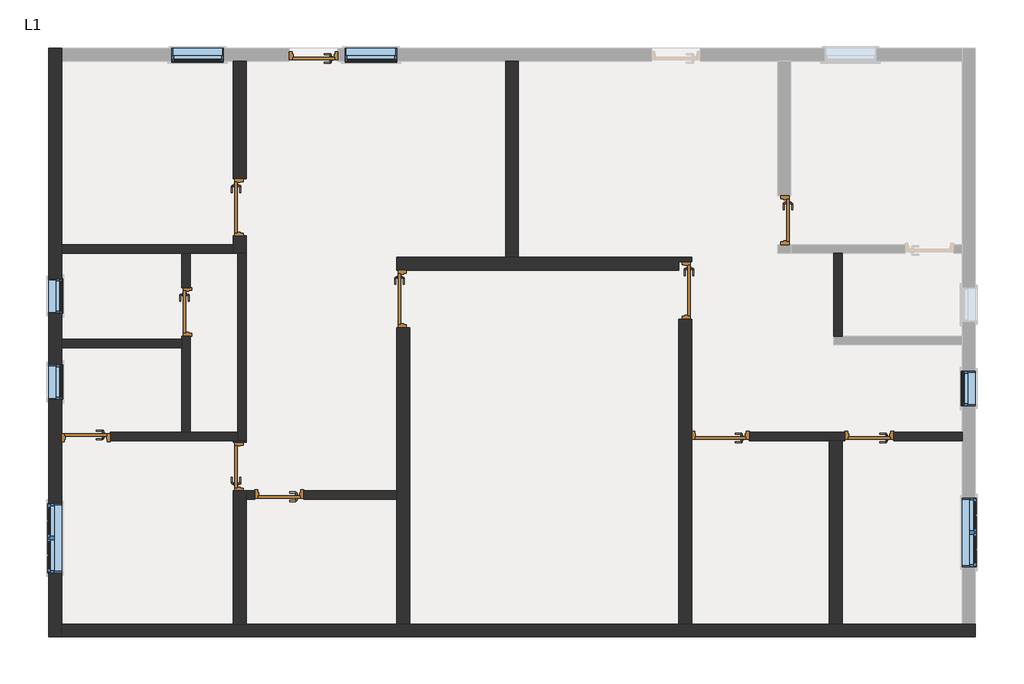
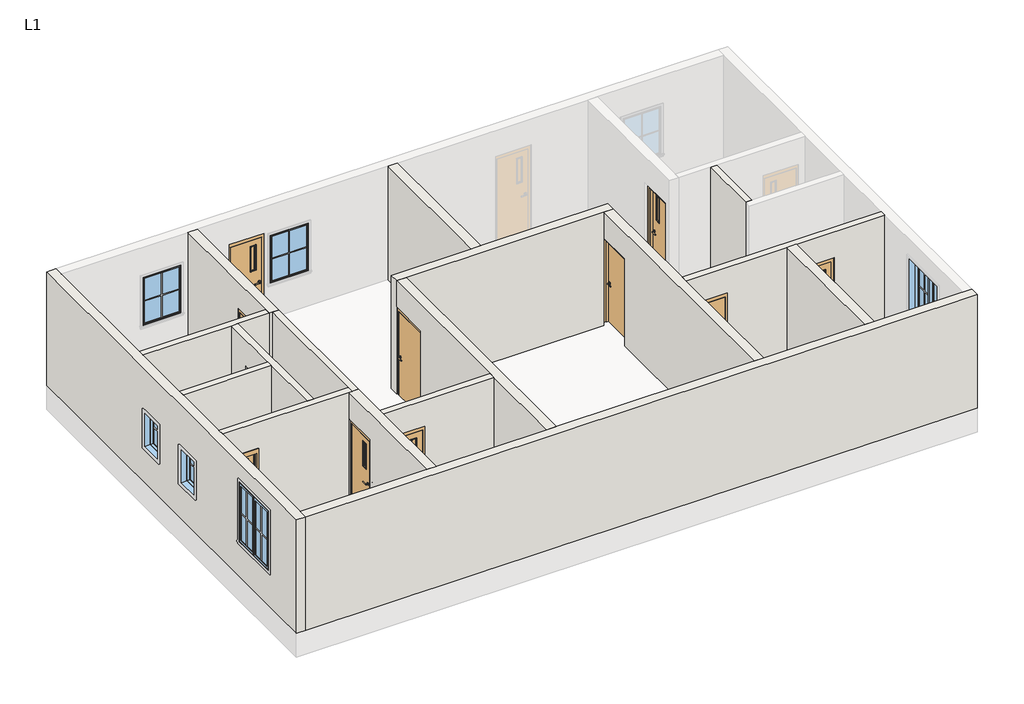
# One storey, part 1 of 2: 17 walls, 11 doors, 7 windows.
"""IFC4 building model written with IfcOpenShell, lengths in millimetres."""

from ifc_helpers import new_model, si_unit, frame, origin, place, context, project, spatial, polyline, outline, extrude, faceted_brep, transform, mapped, element, save
from components import door_9a5ad36a, door_70ceb761, door_9ff278b0, door_e76c17f4, door_2faac2b1, door_21b9ace8, window_8377141f, window_b8e47f08, window_2799360a

model = new_model("IFC4")

# Units and contexts
model_context = context("Model", 3, world=origin())
ifc_project = project(units=[si_unit("LENGTHUNIT", "METRE", prefix="MILLI")], contexts=[model_context])

# Site, building, storey
site = spatial("IfcSite", under=ifc_project)
building = spatial("IfcBuilding", under=site)
storey = spatial("IfcBuildingStorey", under=building, Name="L1", Elevation=609.6)

# Doors
placement = place(None, origin())
door_shape = door_9a5ad36a(model_context)
element("IfcDoor", 1, ObjectType="Door-Passage-Single-Flush : 36\" x 84\"", at=placement, inside=storey, context=model_context, shape_type="MappedRepresentation", body=[
    mapped(door_shape, transform((-2601.2379185, 2629.4278379, 609.6), x_axis=(0.0, -1.0, 0.0), y_axis=(1.0, 0.0, 0.0), z_axis=(0.0, 0.0, 1.0))),
])
element("IfcDoor", 2, ObjectType="Door-Passage-Single-Flush : 36\" x 84\"", at=placement, inside=storey, context=model_context, shape_type="MappedRepresentation", body=[
    mapped(door_shape, transform((294.3620815, 1003.8278379, 609.6), x_axis=(0.0, -1.0, 0.0), y_axis=(1.0, 0.0, 0.0), z_axis=(0.0, 0.0, 1.0))),
])
door_2_shape = door_70ceb761(model_context)
element("IfcDoor", 3, ObjectType="Door-Passage-Single-Flush : 36\" x 84\"", at=placement, inside=storey, context=model_context, shape_type="MappedRepresentation", body=[
    mapped(door_2_shape, transform((5914.1120815, -1428.2221621, 609.6), x_axis=(-1.0, 0.0, 0.0), y_axis=(0.0, -1.0, 0.0), z_axis=(0.0, 0.0, 1.0))),
])
door_3_shape = door_9ff278b0(model_context)
element("IfcDoor", 4, ObjectType="Door-Passage-Single-Flush : 36\" x 84\"", at=placement, inside=storey, context=model_context, shape_type="MappedRepresentation", body=[
    mapped(door_3_shape, transform((5285.4620815, 1156.2278379, 609.6), x_axis=(0.0, -1.0, 0.0), y_axis=(1.0, 0.0, 0.0), z_axis=(0.0, 0.0, 1.0))),
])
door_4_shape = door_e76c17f4(model_context)
element("IfcDoor", 5, ObjectType="Door-Passage-Single-Vision_Lite : 30\" x 84\"", at=placement, inside=storey, context=model_context, shape_type="MappedRepresentation", body=[
    mapped(door_4_shape, transform((-2601.2379185, -1967.9721621, 609.6), x_axis=(0.0, 1.0, 0.0), y_axis=(-1.0, 0.0, 0.0), z_axis=(0.0, 0.0, 1.0))),
])
element("IfcDoor", 6, ObjectType="Door-Passage-Single-Vision_Lite : 30\" x 84\"", at=placement, inside=storey, context=model_context, shape_type="MappedRepresentation", body=[
    mapped(door_4_shape, transform((7038.0620815, 2400.8278379, 609.6), x_axis=(0.0, -1.0, 0.0), y_axis=(1.0, 0.0, 0.0), z_axis=(0.0, 0.0, 1.0))),
])
element("IfcDoor", 7, ObjectType="Door-Passage-Single-Vision_Lite : 30\" x 84\"", at=placement, inside=storey, context=model_context, shape_type="MappedRepresentation", body=[
    mapped(door_4_shape, transform((-1299.4879185, 5340.8778379, 609.6), x_axis=(-1.0, 0.0, 0.0), y_axis=(0.0, -1.0, 0.0), z_axis=(0.0, 0.0, 1.0))),
])
door_5_shape = door_2faac2b1(model_context)
element("IfcDoor", 8, ObjectType="Door-Passage-Single-Vision_Lite : 30\" x 84\"", at=placement, inside=storey, context=model_context, shape_type="MappedRepresentation", body=[
    mapped(door_5_shape, transform((-1909.0879185, -2469.6221621, 609.6), x_axis=(-1.0, 0.0, 0.0), y_axis=(0.0, -1.0, 0.0), z_axis=(0.0, 0.0, 1.0))),
])
element("IfcDoor", 9, ObjectType="Door-Passage-Single-Vision_Lite : 30\" x 84\"", at=placement, inside=storey, context=model_context, shape_type="MappedRepresentation", body=[
    mapped(door_5_shape, transform((8555.7120815, -1428.2221621, 609.6), x_axis=(-1.0, 0.0, 0.0), y_axis=(0.0, -1.0, 0.0), z_axis=(0.0, 0.0, 1.0))),
])
door_6_shape = door_21b9ace8(model_context)
element("IfcDoor", 10, ObjectType="Door-Passage-Single-Vision_Lite : 30\" x 84\"", at=placement, inside=storey, context=model_context, shape_type="MappedRepresentation", body=[
    mapped(door_6_shape, transform((-3553.7379185, 775.2278379, 609.6), x_axis=(0.0, -1.0, 0.0), y_axis=(1.0, 0.0, 0.0), z_axis=(0.0, 0.0, 1.0))),
])
element("IfcDoor", 11, ObjectType="Door-Passage-Single-Vision_Lite : 30\" x 84\"", at=placement, inside=storey, context=model_context, shape_type="MappedRepresentation", body=[
    mapped(door_6_shape, transform((-5338.0879185, -1440.9221621, 609.6), x_axis=(-1.0, 0.0, 0.0), y_axis=(0.0, -1.0, 0.0), z_axis=(0.0, 0.0, 1.0))),
])

# Walls
element("IfcWall", 12, ObjectType="Generic - 6\"", at=placement, inside=storey, context=model_context, shape_type="Brep", body=[
    faceted_brep([(-5769.8879185, 1816.6278379, 609.6), (-3636.2879185, 1816.6278379, 609.6), (-3483.8879185, 1816.6278379, 609.6), (-2721.8879185, 1816.6278379, 609.6), (-2721.8879185, 1816.6278379, 3505.2), (-3483.8879185, 1816.6278379, 3505.2), (-3636.2879185, 1816.6278379, 3505.2), (-5769.8879185, 1816.6278379, 3505.2), (-5769.8879185, 1969.0278379, 609.6), (-5769.8879185, 1969.0278379, 3505.2), (-2721.8879185, 1969.0278379, 3505.2), (-2721.8879185, 1969.0278379, 609.6)], [[[0, 1, 2, 3, 4, 5, 6, 7]], [[8, 9, 10, 11]], [[3, 2, 1, 0, 8, 11]], [[4, 3, 11, 10]], [[0, 7, 9, 8]], [[7, 6, 5, 4, 10, 9]]]),
])
element("IfcWall", 13, ObjectType="Generic - 6\"", at=placement, inside=storey, context=model_context, shape_type="Brep", body=[
    faceted_brep([(-2645.6879185, 1816.6278379, 609.6), (-2645.6879185, -1358.3721621, 609.6), (-2645.6879185, -1510.7721621, 609.6), (-2645.6879185, -1510.7721621, 3505.2), (-2645.6879185, -1358.3721621, 3505.2), (-2645.6879185, 1816.6278379, 3505.2), (-2493.2879185, 1816.6278379, 609.6), (-2493.2879185, 1816.6278379, 3505.2), (-2493.2879185, -1510.7721621, 3505.2), (-2493.2879185, -1510.7721621, 609.6)], [[[0, 1, 2, 3, 4, 5]], [[6, 7, 8, 9]], [[2, 1, 0, 6, 9]], [[0, 5, 7, 6]], [[3, 2, 9, 8]], [[5, 4, 3, 8, 7]]]),
])
element("IfcWall", 14, ObjectType="Generic - 6\"", at=placement, inside=storey, context=model_context, shape_type="Brep", body=[
    faceted_brep([(-2645.6879185, -1358.3721621, 3505.2), (-2645.6879185, -1358.3721621, 609.6), (-3483.8879185, -1358.3721621, 609.6), (-3636.2879185, -1358.3721621, 609.6), (-4906.2879185, -1358.3721621, 609.6), (-4906.2879185, -1358.3721621, 2844.8), (-5769.8879185, -1358.3721621, 2844.8), (-5769.8879185, -1358.3721621, 3505.2), (-3636.2879185, -1358.3721621, 3505.2), (-3483.8879185, -1358.3721621, 3505.2), (-2645.6879185, -1510.7721621, 609.6), (-2645.6879185, -1510.7721621, 3505.2), (-2721.8879185, -1510.7721621, 3505.2), (-5769.8879185, -1510.7721621, 3505.2), (-5769.8879185, -1510.7721621, 2844.8), (-4906.2879185, -1510.7721621, 2844.8), (-4906.2879185, -1510.7721621, 609.6), (-2721.8879185, -1510.7721621, 609.6)], [[[0, 1, 2, 3, 4, 5, 6, 7, 8, 9]], [[10, 11, 12, 13, 14, 15, 16, 17]], [[1, 10, 17, 16, 4, 3, 2]], [[1, 0, 11, 10]], [[13, 7, 6, 14]], [[5, 15, 14, 6]], [[15, 5, 4, 16]], [[0, 9, 8, 7, 13, 12, 11]]]),
])
element("IfcWall", 15, ObjectType="Generic - 6\"", at=placement, inside=storey, context=model_context, shape_type="Brep", body=[
    faceted_brep([(173.7120815, -2552.1721621, 609.6), (173.7120815, -2552.1721621, 3505.2), (-2493.2879185, -2552.1721621, 3505.2), (-2493.2879185, -2552.1721621, 609.6), (-2340.8879185, -2552.1721621, 609.6), (-2340.8879185, -2552.1721621, 2844.8), (-1477.2879185, -2552.1721621, 2844.8), (-1477.2879185, -2552.1721621, 609.6), (173.7120815, -2399.7721621, 3505.2), (173.7120815, -2399.7721621, 609.6), (-1477.2879185, -2399.7721621, 609.6), (-1477.2879185, -2399.7721621, 2844.8), (-2340.8879185, -2399.7721621, 2844.8), (-2340.8879185, -2399.7721621, 609.6), (-2493.2879185, -2399.7721621, 609.6), (-2493.2879185, -2399.7721621, 2844.8), (-2493.2879185, -2399.7721621, 3505.2)], [[[0, 1, 2, 3, 4, 5, 6, 7]], [[8, 9, 10, 11, 12, 13, 14, 15, 16]], [[3, 14, 13, 4]], [[9, 0, 7, 10]], [[1, 0, 9, 8]], [[3, 2, 16, 15, 14]], [[12, 5, 4, 13]], [[5, 12, 11, 6]], [[6, 11, 10, 7]], [[2, 1, 8, 16]]]),
])
element("IfcWall", 16, ObjectType="Generic - 6\"", at=placement, inside=storey, context=model_context, shape_type="SweptSolid", body=[
    extrude(outline(polyline([(609.6, 10206.7120815), (3505.2, 10206.7120815), (3505.2, 5406.1120815), (2844.8, 5406.1120815), (2844.8, 6422.1120815), (609.6, 6422.1120815), (609.6, 8123.9120815), (2844.8, 8123.9120815), (2844.8, 8987.5120815), (609.6, 8987.5120815), (609.6, 10206.7120815)])), frame((0.0, -1510.7721621, 0.0), z_axis=(0.0, 1.0, 0.0), x_axis=(0.0, 0.0, 1.0)), (0.0, 0.0, 1.0), 152.4),
])
element("IfcWall", 17, ObjectType="Generic - 6\"", at=placement, inside=storey, context=model_context, shape_type="SweptSolid", body=[
    extrude(outline(polyline([(8073.1120815, 1816.6278379), (8073.1120815, 343.4278379), (7920.7120815, 343.4278379), (7920.7120815, 1816.6278379), (8073.1120815, 1816.6278379)])), frame((0.0, 0.0, 609.6), z_axis=(0.0, 0.0, 1.0), x_axis=(1.0, 0.0, 0.0)), (0.0, 0.0, 1.0), 2895.6),
])
element("IfcWall", 18, ObjectType="Generic - 6\"", at=placement, inside=storey, context=model_context, shape_type="Brep", body=[
    faceted_brep([(-3636.2879185, 1816.6278379, 3505.2), (-3636.2879185, 1816.6278379, 609.6), (-3636.2879185, 1207.0278379, 609.6), (-3636.2879185, 1207.0278379, 2844.8), (-3636.2879185, 343.4278379, 2844.8), (-3636.2879185, 343.4278379, 609.6), (-3636.2879185, 292.6278379, 609.6), (-3636.2879185, 140.2278379, 609.6), (-3636.2879185, -1358.3721621, 609.6), (-3636.2879185, -1358.3721621, 3505.2), (-3636.2879185, 140.2278379, 3505.2), (-3636.2879185, 292.6278379, 3505.2), (-3483.8879185, 1816.6278379, 609.6), (-3483.8879185, 1816.6278379, 3505.2), (-3483.8879185, -1358.3721621, 3505.2), (-3483.8879185, -1358.3721621, 609.6), (-3483.8879185, 343.4278379, 609.6), (-3483.8879185, 343.4278379, 2844.8), (-3483.8879185, 1207.0278379, 2844.8), (-3483.8879185, 1207.0278379, 609.6)], [[[0, 1, 2, 3, 4, 5, 6, 7, 8, 9, 10, 11]], [[12, 13, 14, 15, 16, 17, 18, 19]], [[1, 12, 19, 2]], [[15, 8, 7, 6, 5, 16]], [[1, 0, 13, 12]], [[9, 8, 15, 14]], [[4, 17, 16, 5]], [[17, 4, 3, 18]], [[18, 3, 2, 19]], [[0, 11, 10, 9, 14, 13]]]),
])
element("IfcWall", 19, ObjectType="Generic - 6\"", at=placement, inside=storey, context=model_context, shape_type="SweptSolid", body=[
    extrude(outline(polyline([(-3636.2879185, 140.2278379), (-5769.8879185, 140.2278379), (-5769.8879185, 292.6278379), (-3636.2879185, 292.6278379), (-3636.2879185, 140.2278379)])), frame((0.0, 0.0, 609.6), z_axis=(0.0, 0.0, 1.0), x_axis=(1.0, 0.0, 0.0)), (0.0, 0.0, 1.0), 2895.6),
])
element("IfcWall", 20, ObjectType="Generic - 9\"", at=placement, inside=storey, context=model_context, shape_type="Brep", body=[
    faceted_brep([(-5998.4879185, 5448.8278379, 609.6), (-5998.4879185, -4990.5721621, 609.6), (-5998.4879185, -4990.5721621, 3505.2), (-5998.4879185, 5448.8278379, 3505.2), (-5998.4879185, -774.1721621, 2438.4), (-5998.4879185, -774.1721621, 1524.0), (-5998.4879185, -164.5721621, 1524.0), (-5998.4879185, -164.5721621, 2438.4), (-5998.4879185, 749.8278379, 2438.4), (-5998.4879185, 749.8278379, 1524.0), (-5998.4879185, 1359.4278379, 1524.0), (-5998.4879185, 1359.4278379, 2438.4), (-5998.4879185, -2628.3721621, 1524.0), (-5998.4879185, -2628.3721621, 3048.0), (-5998.4879185, -3847.5721621, 3048.0), (-5998.4879185, -3847.5721621, 1524.0), (-5769.8879185, -4990.5721621, 609.6), (-5769.8879185, -4761.9721621, 609.6), (-5769.8879185, -1510.7721621, 609.6), (-5769.8879185, -1358.3721621, 609.6), (-5769.8879185, 140.2278379, 609.6), (-5769.8879185, 292.6278379, 609.6), (-5769.8879185, 1816.6278379, 609.6), (-5769.8879185, 1969.0278379, 609.6), (-5769.8879185, 5220.2278379, 609.6), (-5769.8879185, 5448.8278379, 609.6), (-5769.8879185, 5448.8278379, 3505.2), (-5769.8879185, 5220.2278379, 3505.2), (-5769.8879185, 1969.0278379, 3505.2), (-5769.8879185, 1816.6278379, 3505.2), (-5769.8879185, 292.6278379, 3505.2), (-5769.8879185, 140.2278379, 3505.2), (-5769.8879185, -1358.3721621, 3505.2), (-5769.8879185, -1510.7721621, 3505.2), (-5769.8879185, -4761.9721621, 3505.2), (-5769.8879185, -4990.5721621, 3505.2), (-5769.8879185, -774.1721621, 2438.4), (-5769.8879185, -164.5721621, 2438.4), (-5769.8879185, -164.5721621, 1524.0), (-5769.8879185, -774.1721621, 1524.0), (-5769.8879185, 749.8278379, 2438.4), (-5769.8879185, 1359.4278379, 2438.4), (-5769.8879185, 1359.4278379, 1524.0), (-5769.8879185, 749.8278379, 1524.0), (-5769.8879185, -2628.3721621, 3048.0), (-5769.8879185, -2628.3721621, 1524.0), (-5769.8879185, -3847.5721621, 1524.0), (-5769.8879185, -3847.5721621, 3048.0)], [[[0, 1, 2, 3], [4, 5, 6, 7], [8, 9, 10, 11], [12, 13, 14, 15]], [[16, 17, 18, 19, 20, 21, 22, 23, 24, 25, 26, 27, 28, 29, 30, 31, 32, 33, 34, 35], [36, 37, 38, 39], [40, 41, 42, 43], [44, 45, 46, 47]], [[1, 0, 25, 24, 23, 22, 21, 20, 19, 18, 17, 16]], [[2, 1, 16, 35]], [[0, 3, 26, 25]], [[5, 4, 36, 39]], [[6, 5, 39, 38]], [[7, 6, 38, 37]], [[4, 7, 37, 36]], [[9, 8, 40, 43]], [[10, 9, 43, 42]], [[11, 10, 42, 41]], [[8, 11, 41, 40]], [[3, 2, 35, 34, 33, 32, 31, 30, 29, 28, 27, 26]], [[44, 13, 12, 45]], [[45, 12, 15, 46]], [[46, 15, 14, 47]], [[13, 44, 47, 14]]]),
])
element("IfcWall", 21, ObjectType="Generic - 9\"", at=placement, inside=storey, context=model_context, shape_type="Brep", body=[
    faceted_brep([(-5769.8879185, -4990.5721621, 609.6), (10435.3120815, -4990.5721621, 609.6), (10435.3120815, -4990.5721621, 3505.2), (-5769.8879185, -4990.5721621, 3505.2), (-5769.8879185, -4761.9721621, 609.6), (-5769.8879185, -4761.9721621, 3505.2), (-2721.8879185, -4761.9721621, 3505.2), (-2493.2879185, -4761.9721621, 3505.2), (173.7120815, -4761.9721621, 3505.2), (402.3120815, -4761.9721621, 3505.2), (5177.5120815, -4761.9721621, 3505.2), (5406.1120815, -4761.9721621, 3505.2), (7844.5120815, -4761.9721621, 3505.2), (8073.1120815, -4761.9721621, 3505.2), (10206.7120815, -4761.9721621, 3505.2), (10435.3120815, -4761.9721621, 3505.2), (10435.3120815, -4761.9721621, 609.6), (10206.7120815, -4761.9721621, 609.6), (8073.1120815, -4761.9721621, 609.6), (7844.5120815, -4761.9721621, 609.6), (5406.1120815, -4761.9721621, 609.6), (5177.5120815, -4761.9721621, 609.6), (402.3120815, -4761.9721621, 609.6), (173.7120815, -4761.9721621, 609.6), (-2493.2879185, -4761.9721621, 609.6), (-2721.8879185, -4761.9721621, 609.6)], [[[0, 1, 2, 3]], [[4, 5, 6, 7, 8, 9, 10, 11, 12, 13, 14, 15, 16, 17, 18, 19, 20, 21, 22, 23, 24, 25]], [[1, 0, 4, 25, 24, 23, 22, 21, 20, 19, 18, 17, 16]], [[0, 3, 5, 4]], [[2, 1, 16, 15]], [[3, 2, 15, 14, 13, 12, 11, 10, 9, 8, 7, 6, 5]]]),
])
element("IfcWall", 22, ObjectType="Generic - 9\"", at=placement, inside=storey, context=model_context, shape_type="Brep", body=[
    faceted_brep([(-2721.8879185, 5220.2278379, 3505.2), (-2721.8879185, 5220.2278379, 609.6), (-2721.8879185, 3137.4278379, 609.6), (-2721.8879185, 3137.4278379, 2844.8), (-2721.8879185, 2121.4278379, 2844.8), (-2721.8879185, 2121.4278379, 609.6), (-2721.8879185, 1969.0278379, 609.6), (-2721.8879185, 1816.6278379, 609.6), (-2721.8879185, 1816.6278379, 3505.2), (-2721.8879185, 1969.0278379, 3505.2), (-2493.2879185, 5220.2278379, 609.6), (-2493.2879185, 5220.2278379, 3505.2), (-2493.2879185, 1816.6278379, 3505.2), (-2493.2879185, 1816.6278379, 609.6), (-2493.2879185, 2121.4278379, 609.6), (-2493.2879185, 2121.4278379, 2844.8), (-2493.2879185, 3137.4278379, 2844.8), (-2493.2879185, 3137.4278379, 609.6), (-2645.6879185, 1816.6278379, 609.6), (-2645.6879185, 1816.6278379, 3505.2)], [[[0, 1, 2, 3, 4, 5, 6, 7, 8, 9]], [[10, 11, 12, 13, 14, 15, 16, 17]], [[1, 10, 17, 2]], [[13, 18, 7, 6, 5, 14]], [[1, 0, 11, 10]], [[8, 7, 18, 13, 12, 19]], [[4, 15, 14, 5]], [[15, 4, 3, 16]], [[16, 3, 2, 17]], [[0, 9, 8, 19, 12, 11]]]),
])
element("IfcWall", 23, ObjectType="Generic - 9\"", at=placement, inside=storey, context=model_context, shape_type="SweptSolid", body=[
    extrude(outline(polyline([(2104.1120815, 1740.4278379), (2104.1120815, 5220.2278379), (2332.7120815, 5220.2278379), (2332.7120815, 1740.4278379), (2104.1120815, 1740.4278379)])), frame((0.0, 0.0, 609.6), z_axis=(0.0, 0.0, 1.0), x_axis=(1.0, 0.0, 0.0)), (0.0, 0.0, 1.0), 2895.6),
])
element("IfcWall", 24, ObjectType="Generic - 9\"", at=placement, inside=storey, context=model_context, shape_type="Brep", body=[
    faceted_brep([(173.7120815, 1511.8278379, 3505.2), (173.7120815, 1511.8278379, 2844.8), (173.7120815, 1511.8278379, 609.6), (5177.5120815, 1511.8278379, 609.6), (5177.5120815, 1511.8278379, 2844.8), (5406.1120815, 1511.8278379, 2844.8), (5406.1120815, 1511.8278379, 3505.2), (5177.5120815, 1511.8278379, 3505.2), (402.3120815, 1511.8278379, 3505.2), (5406.1120815, 1740.4278379, 609.6), (2332.7120815, 1740.4278379, 609.6), (2104.1120815, 1740.4278379, 609.6), (173.7120815, 1740.4278379, 609.6), (173.7120815, 1740.4278379, 3505.2), (2104.1120815, 1740.4278379, 3505.2), (2332.7120815, 1740.4278379, 3505.2), (5406.1120815, 1740.4278379, 3505.2), (5406.1120815, 1664.2278379, 609.6), (5177.5120815, 1664.2278379, 609.6), (5406.1120815, 1664.2278379, 2844.8), (5177.5120815, 1664.2278379, 2844.8)], [[[0, 1, 2, 3, 4, 5, 6, 7, 8]], [[9, 10, 11, 12, 13, 14, 15, 16]], [[12, 11, 10, 9, 17, 18, 3, 2]], [[9, 16, 6, 5, 19, 17]], [[2, 1, 0, 13, 12]], [[18, 20, 4, 3]], [[20, 19, 5, 4]], [[20, 18, 17, 19]], [[0, 8, 7, 6, 16, 15, 14, 13]]]),
])
element("IfcWall", 25, ObjectType="Generic - 9\"", at=placement, inside=storey, context=model_context, shape_type="SweptSolid", body=[
    extrude(outline(polyline([(8073.1120815, -1512.0421621), (8073.1120815, -4761.9721621), (7844.5120815, -4761.9721621), (7844.5120815, -1512.0421621), (8073.1120815, -1512.0421621)])), frame((0.0, 0.0, 609.6), z_axis=(0.0, 0.0, 1.0), x_axis=(1.0, 0.0, 0.0)), (0.0, 0.0, 1.0), 2895.6),
])
element("IfcWall", 26, ObjectType="Generic - 9\"", at=placement, inside=storey, context=model_context, shape_type="Brep", body=[
    faceted_brep([(5406.1120815, -4761.9721621, 3505.2), (5406.1120815, -4761.9721621, 609.6), (5406.1120815, -1510.7721621, 609.6), (5406.1120815, -1358.3721621, 609.6), (5406.1120815, 648.2278379, 609.6), (5406.1120815, 648.2278379, 2844.8), (5406.1120815, 1511.8278379, 2844.8), (5406.1120815, 1511.8278379, 3505.2), (5406.1120815, -1358.3721621, 3505.2), (5406.1120815, -1510.7721621, 3505.2), (5177.5120815, -4761.9721621, 609.6), (5177.5120815, -4761.9721621, 3505.2), (5177.5120815, 1511.8278379, 3505.2), (5177.5120815, 1511.8278379, 2844.8), (5177.5120815, 648.2278379, 2844.8), (5177.5120815, 648.2278379, 609.6)], [[[0, 1, 2, 3, 4, 5, 6, 7, 8, 9]], [[10, 11, 12, 13, 14, 15]], [[1, 10, 15, 4, 3, 2]], [[12, 7, 6, 13]], [[1, 0, 11, 10]], [[14, 5, 4, 15]], [[5, 14, 13, 6]], [[0, 9, 8, 7, 12, 11]]]),
])
element("IfcWall", 27, ObjectType="Generic - 9\"", at=placement, inside=storey, context=model_context, shape_type="Brep", body=[
    faceted_brep([(402.3120815, -4761.9721621, 3505.2), (402.3120815, -4761.9721621, 609.6), (402.3120815, 495.8278379, 609.6), (402.3120815, 495.8278379, 2844.8), (402.3120815, 1511.8278379, 2844.8), (402.3120815, 1511.8278379, 3505.2), (173.7120815, -4761.9721621, 609.6), (173.7120815, -4761.9721621, 3505.2), (173.7120815, -2552.1721621, 3505.2), (173.7120815, -2399.7721621, 3505.2), (173.7120815, 1511.8278379, 3505.2), (173.7120815, 1511.8278379, 2844.8), (173.7120815, 495.8278379, 2844.8), (173.7120815, 495.8278379, 609.6), (173.7120815, -2399.7721621, 609.6), (173.7120815, -2552.1721621, 609.6)], [[[0, 1, 2, 3, 4, 5]], [[6, 7, 8, 9, 10, 11, 12, 13, 14, 15]], [[1, 6, 15, 14, 13, 2]], [[10, 5, 4, 11]], [[1, 0, 7, 6]], [[12, 3, 2, 13]], [[3, 12, 11, 4]], [[0, 5, 10, 9, 8, 7]]]),
])
element("IfcWall", 28, ObjectType="Generic - 9\"", at=placement, inside=storey, context=model_context, shape_type="Brep", body=[
    faceted_brep([(-2493.2879185, -4761.9721621, 3505.2), (-2493.2879185, -4761.9721621, 609.6), (-2493.2879185, -2552.1721621, 609.6), (-2493.2879185, -2399.7721621, 609.6), (-2493.2879185, -2399.7721621, 2844.8), (-2493.2879185, -1536.1721621, 2844.8), (-2493.2879185, -1536.1721621, 609.6), (-2493.2879185, -1510.7721621, 609.6), (-2493.2879185, -1510.7721621, 3505.2), (-2493.2879185, -2399.7721621, 3505.2), (-2493.2879185, -2552.1721621, 3505.2), (-2721.8879185, -4761.9721621, 609.6), (-2721.8879185, -4761.9721621, 3505.2), (-2721.8879185, -1510.7721621, 3505.2), (-2721.8879185, -1510.7721621, 609.6), (-2721.8879185, -1536.1721621, 609.6), (-2721.8879185, -1536.1721621, 2844.8), (-2721.8879185, -2399.7721621, 2844.8), (-2721.8879185, -2399.7721621, 609.6), (-2645.6879185, -1510.7721621, 609.6), (-2645.6879185, -1510.7721621, 3505.2)], [[[0, 1, 2, 3, 4, 5, 6, 7, 8, 9, 10]], [[11, 12, 13, 14, 15, 16, 17, 18]], [[1, 11, 18, 3, 2]], [[14, 19, 7, 6, 15]], [[1, 0, 12, 11]], [[8, 7, 19, 14, 13, 20]], [[5, 16, 15, 6]], [[16, 5, 4, 17]], [[17, 4, 3, 18]], [[0, 10, 9, 8, 20, 13, 12]]]),
])

# Windows
window_shape = window_8377141f(model_context)
element("IfcWindow", 29, ObjectType="Window-Casement-Double : 48\" x 60\"", at=placement, inside=storey, context=model_context, shape_type="MappedRepresentation", body=[
    mapped(window_shape, transform((10321.0120815, -3136.3721621, 609.6), x_axis=(0.0, -1.0, 0.0), y_axis=(1.0, 0.0, 0.0), z_axis=(0.0, 0.0, 1.0))),
])
element("IfcWindow", 30, ObjectType="Window-Casement-Double : 48\" x 60\"", at=placement, inside=storey, context=model_context, shape_type="MappedRepresentation", body=[
    mapped(window_shape, transform((-5884.1879185, -3237.9721621, 609.6), x_axis=(0.0, 1.0, 0.0), y_axis=(-1.0, 0.0, 0.0), z_axis=(0.0, 0.0, 1.0))),
])
window_2_shape = window_b8e47f08(model_context)
element("IfcWindow", 31, ObjectType="Window-Fixed : 24\" x 36\"", at=placement, inside=storey, context=model_context, shape_type="MappedRepresentation", body=[
    mapped(window_2_shape, transform((-5884.1879185, -469.3721621, 609.6), x_axis=(0.0, -1.0, 0.0), y_axis=(1.0, 0.0, 0.0), z_axis=(0.0, 0.0, 1.0))),
])
element("IfcWindow", 32, ObjectType="Window-Fixed : 24\" x 36\"", at=placement, inside=storey, context=model_context, shape_type="MappedRepresentation", body=[
    mapped(window_2_shape, transform((-5884.1879185, 1054.6278379, 609.6), x_axis=(0.0, -1.0, 0.0), y_axis=(1.0, 0.0, 0.0), z_axis=(0.0, 0.0, 1.0))),
])
element("IfcWindow", 33, ObjectType="Window-Fixed : 24\" x 36\"", at=placement, inside=storey, context=model_context, shape_type="MappedRepresentation", body=[
    mapped(window_2_shape, transform((10321.0120815, -583.6721621, 609.6), x_axis=(0.0, 1.0, 0.0), y_axis=(-1.0, 0.0, 0.0), z_axis=(0.0, 0.0, 1.0))),
])
window_3_shape = window_2799360a(model_context)
element("IfcWindow", 34, ObjectType="Window-Fixed : 36\" x 48\"", at=placement, inside=storey, context=model_context, shape_type="MappedRepresentation", body=[
    mapped(window_3_shape, transform((-3356.8879185, 5334.5278379, 609.6), x_axis=(-1.0, 0.0, 0.0), y_axis=(0.0, -1.0, 0.0), z_axis=(0.0, 0.0, 1.0))),
])
element("IfcWindow", 35, ObjectType="Window-Fixed : 36\" x 48\"", at=placement, inside=storey, context=model_context, shape_type="MappedRepresentation", body=[
    mapped(window_3_shape, transform((-283.4879185, 5334.5278379, 609.6), x_axis=(-1.0, 0.0, 0.0), y_axis=(0.0, -1.0, 0.0), z_axis=(0.0, 0.0, 1.0))),
])

save(model, "model.ifc")

# Revit data of these elements
# Type "Door-Passage-Single-Flush : 36\" x 84\""
#   Type Mark = "11"
#   Assembly Code = "B2030200"
#   Analytic Construction = "Wooden"
#   Thickness = 0' - 1 3/4"
#   Thermal Resistance (R) = 2.5876 (h·ft²·°F)/BTU
#   Swing Angle [instance default] = 90.00°
#   Strike Height = 3' - 4"
#   Rough Width [instance default] = 3' - 4"
#   Rough Height [instance default] = 7' - 4"
#   MF Opening Height [instance default] = 0' - 4"
#   MF Opening Width [instance default] = 0' - 4"
#   Inset Calculate [instance default] = 0' - 4"
#   Masonry Inset [instance default] = 0' - 1"
#   Height = 7' - 0"
#   Width = 3' - 0"
#   Heat Transfer Coefficient (U) = 0.3865 BTU/(h·ft²·°F)
#   Masonry Frame Depth = 0' - 5 3/4"
#   Masonry Frame [instance default] = yes
#   Function = 1
#   Dry Wall Frame [instance default] = no
#   Define Thermal Properties by = 1
#   Panel Material = Wood - Birch
#   Frame Material = Metal - Paint Finish - Grey
#   Door Handle Material = Aluminum
#   Visual Light Transmittance = 0
#   Solar Heat Gain Coefficient = 0
#   Wall Closure = (empty or 0)
# Type "Door-Passage-Single-Vision_Lite : 30\" x 84\""
#   Type Mark = "20"
#   Assembly Code = "B2030100"
#   Analytic Construction = "Wooden"
#   Thickness = 0' - 1 3/4"
#   Thermal Resistance (R) = 2.5876 (h·ft²·°F)/BTU
#   Swing Angle [instance default] = 90.00°
#   Strike Height = 3' - 4"
#   Rough Width [instance default] = 2' - 10"
#   Rough Height [instance default] = 7' - 4"
#   MFOpeningHeight [instance default] = 0' - 4"
#   MFOpeningWidth [instance default] = 0' - 4"
#   Inset Calculate [instance default] = 0' - 4"
#   Masonry Inset [instance default] = 0' - 1"
#   Height = 7' - 0"
#   Width = 2' - 6"
#   Heat Transfer Coefficient (U) = 0.3865 BTU/(h·ft²·°F)
#   Masonry Frame Depth = 0' - 5 3/4"
#   Masonry Frame [instance default] = yes
#   Function = 1
#   Dry Wall Frame [instance default] = no
#   Define Thermal Properties by = 1
#   Panel Material = Wood - Birch
#   Glazing = Glass
#   Glass Stop Material = Metal - Paint Finish - Grey
#   Frame Material = Metal - Paint Finish - Grey
#   Door Handle Material = Aluminum
#   Visual Light Transmittance = 0
#   Solar Heat Gain Coefficient = 0
#   Wall Closure = (empty or 0)
# Type "Generic - 6\""
#   Description = "Generic Wall (Material By Category), 6\" thick"
#   Assembly Code = "B2010"
#   Type Mark = "G04"
#   Layers, outside or top first: 0' - 6" no material (function 1)
# Type "Generic - 9\""
#   Description = "Generic Wall (Material By Category), 8\" thick"
#   Assembly Code = "B2010"
#   Type Mark = "G06"
#   Layers, outside or top first: 0' - 9" no material (function 1)
# Type "Window-Casement-Double : 48\" x 60\""
#   Type Mark = "16"
#   Fire Rating = "0.5h"
#   Assembly Code = "B2020100"
#   Analytic Construction = "Double glazing - domestic"
#   Frame Extension [instance default] = 0' - 0 1/4"
#   Window Inset [instance default] = 0' - 0"
#   Wall Thickness [instance default] = 0' - 6"
#   Interior Wall Closure [instance default] = 0' - 2 1/4"
#   Half Width = 2' - 0"
#   Visual Light Transmittance = 0.81
#   Thermal Resistance (R) = 1.8146 (h·ft²·°F)/BTU
#   Solar Heat Gain Coefficient = 0.76
#   Rough Width = 4' - 0 1/2"
#   Rough Height = 5' - 0 1/2"
#   Height = 5' - 0"
#   Heat Transfer Coefficient (U) = 0.5511 BTU/(h·ft²·°F)
#   Exterior Wall Closure [instance default] = 0' - 1 1/4"
#   Extension Jamb [instance default] = 0' - 2 1/4"
#   Default Sill Height = 3' - 0"
#   Width = 4' - 0"
#   Define Thermal Properties by = 0
#   Muntin Visibility = yes
#   Interior Trim Visibility [instance default] = yes
#   Exterior Trim Visibility [instance default] = yes
#   Extension Jamb Visibility [instance default] = yes
#   Interior Trim Material = Wood - Stained
#   Muntin Pattern = Muntin Pattern_2x2 : Muntin Pattern_2x2
#   Interior Trim = Trim-Window-Interior-Flat : Picture Frame
#   Interior Frame Material = Wood - Stained
#   Glass Panel Material = Glass
#   Exterior Trim Material = Clad - White
#   Exterior Trim = Trim-Window-Exterior-Flat : with Sill
#   Exterior Frame Material = Clad - White
#   Define Thermal Properties by = (empty or 0)
#   Wall Closure = (empty or 0)
# Type "Window-Fixed : 24\" x 36\""
#   Type Mark = "18"
#   Fire Rating = "0.5h"
#   Assembly Code = "B2020100"
#   Analytic Construction = "Double glazing - domestic"
#   Window Inset [instance default] = 0' - 0"
#   Wall Thickness [instance default] = 0' - 6"
#   Visual Light Transmittance = 0.81
#   Thermal Resistance (R) = 1.8146 (h·ft²·°F)/BTU
#   Solar Heat Gain Coefficient = 0.76
#   Rough Width = 2' - 0 1/2"
#   Rough Height = 3' - 0 1/2"
#   Interior Wall Closure [instance default] = 0' - 2 1/4"
#   Height = 3' - 0"
#   Heat Transfer Coefficient (U) = 0.5511 BTU/(h·ft²·°F)
#   Frame Extension [instance default] = 0' - 0 1/4"
#   Exterior Wall Closure [instance default] = 0' - 1 1/4"
#   Extension Jamb [instance default] = 0' - 2 1/4"
#   Default Sill Height = 3' - 0"
#   Width = 2' - 0"
#   Muntin Visibility = yes
#   Interior Trim Visibility [instance default] = yes
#   Exterior Trim Visibility [instance default] = yes
#   Extension Jamb Visibility [instance default] = yes
#   Define Thermal Properties by = 1
#   Muntin Pattern = Muntin Pattern_2x2 : Muntin Pattern_2x2
#   Interior Trim Material = Wood - Stained
#   Interior Trim = Trim-Window-Interior-Flat : Picture Frame
#   Interior Frame Material = Wood - Stained
#   Glass Panel Material = Glass
#   Exterior Trim Material = Clad - White
#   Exterior Trim = Trim-Window-Exterior-Flat : with Sill
#   Exterior Frame Material = Clad - White
#   Wall Closure = (empty or 0)
# Type "Window-Fixed : 36\" x 48\""
#   Type Mark = "22"
#   Fire Rating = "0.5h"
#   Assembly Code = "B2020100"
#   Analytic Construction = "Double glazing - domestic"
#   Window Inset [instance default] = 0' - 0"
#   Wall Thickness [instance default] = 0' - 6"
#   Visual Light Transmittance = 0.81
#   Thermal Resistance (R) = 1.8146 (h·ft²·°F)/BTU
#   Solar Heat Gain Coefficient = 0.76
#   Rough Width = 3' - 0 1/2"
#   Rough Height = 4' - 0 1/2"
#   Interior Wall Closure [instance default] = 0' - 2 1/4"
#   Height = 4' - 0"
#   Heat Transfer Coefficient (U) = 0.5511 BTU/(h·ft²·°F)
#   Frame Extension [instance default] = 0' - 0 1/4"
#   Exterior Wall Closure [instance default] = 0' - 1 1/4"
#   Extension Jamb [instance default] = 0' - 2 1/4"
#   Default Sill Height = 3' - 0"
#   Width = 3' - 0"
#   Muntin Visibility = yes
#   Interior Trim Visibility [instance default] = yes
#   Exterior Trim Visibility [instance default] = yes
#   Extension Jamb Visibility [instance default] = yes
#   Define Thermal Properties by = 1
#   Muntin Pattern = Muntin Pattern_2x2 : Muntin Pattern_2x2
#   Interior Trim Material = Wood - Stained
#   Interior Trim = Trim-Window-Interior-Flat : Picture Frame
#   Interior Frame Material = Wood - Stained
#   Glass Panel Material = Glass
#   Exterior Trim Material = Clad - White
#   Exterior Trim = Trim-Window-Exterior-Flat : with Sill
#   Exterior Frame Material = Clad - White
#   Wall Closure = (empty or 0)
# Elements 1, 2, 3, 4 (IfcDoor, "Door-Passage-Single-Flush : 36\" x 84\"")
#   Swing Angle = 90.00°
#   Rough Width = 3' - 4"
#   Rough Height = 7' - 4"
#   Masonry Inset = 0' - 1"
#   MF Opening Width = 0' - 4"
#   MF Opening Height = 0' - 4"
#   Inset Calculate = 0' - 4"
#   Masonry Frame = yes
#   Dry Wall Frame = no
#   Phase Created = New Construction
#   Materials on its faces: "Aluminum", "Metal - Paint Finish - Grey", "Wood - Birch"
# Elements 5, 6, 7, 8, 9, 10, 11 (IfcDoor, "Door-Passage-Single-Vision_Lite : 30\" x 84\"")
#   Swing Angle = 90.00°
#   Rough Width = 2' - 10"
#   Rough Height = 7' - 4"
#   Masonry Inset = 0' - 1"
#   MFOpeningWidth = 0' - 4"
#   MFOpeningHeight = 0' - 4"
#   Inset Calculate = 0' - 4"
#   Masonry Frame = yes
#   Dry Wall Frame = no
#   Phase Created = New Construction
#   Materials on its faces: "Metal - Paint Finish - Grey", "Aluminum", "Wood - Birch", "Glass"
# Elements 12, 13, 14, 15, 16, 17, 18, 19 (IfcWall, "Generic - 6\"")
#   Top Offset = 0' - 0"
#   Base Offset = 0' - 0"
#   wall height = 9' - 6"
#   Phase Created = New Construction
#   Base Constraint = L1
#   Top Constraint = L2
#   Materials on its faces: "Default Wall"
# Elements 20, 21, 22, 23, 24, 25, 26, 27, 28 (IfcWall, "Generic - 9\"")
#   Top Offset = 0' - 0"
#   Base Offset = 0' - 0"
#   wall height = 9' - 6"
#   Phase Created = New Construction
#   Base Constraint = L1
#   Top Constraint = L2
#   Materials on its faces: "Default Wall"
# Element 29 (IfcWindow, "Window-Casement-Double : 48\" x 60\"")
#   Mark = "107"
#   Window Inset = 0' - 0"
#   Interior Wall Closure = 0' - 2 1/4"
#   Frame Extension = 0' - 0 1/4"
#   Exterior Wall Closure = 0' - 1 1/4"
#   Interior Trim Visibility = yes
#   Exterior Trim Visibility = yes
#   Phase Created = New Construction
#   Materials on its faces: "Wood - Stained", "Glass", "Clad - White"
# Element 30 (IfcWindow, "Window-Casement-Double : 48\" x 60\"")
#   Mark = "108"
#   Window Inset = 0' - 0"
#   Interior Wall Closure = 0' - 2 1/4"
#   Frame Extension = 0' - 0 1/4"
#   Exterior Wall Closure = 0' - 1 1/4"
#   Interior Trim Visibility = yes
#   Exterior Trim Visibility = yes
#   Phase Created = New Construction
#   Materials on its faces: "Wood - Stained", "Glass", "Clad - White"
# Element 31 (IfcWindow, "Window-Fixed : 24\" x 36\"")
#   Mark = "103"
#   Window Inset = 0' - 0"
#   Interior Wall Closure = 0' - 2 1/4"
#   Frame Extension = 0' - 0 1/4"
#   Exterior Wall Closure = 0' - 1 1/4"
#   Interior Trim Visibility = yes
#   Exterior Trim Visibility = yes
#   Phase Created = New Construction
#   Materials on its faces: "Wood - Stained", "Glass", "Clad - White"
# Element 32 (IfcWindow, "Window-Fixed : 24\" x 36\"")
#   Mark = "104"
#   Window Inset = 0' - 0"
#   Interior Wall Closure = 0' - 2 1/4"
#   Frame Extension = 0' - 0 1/4"
#   Exterior Wall Closure = 0' - 1 1/4"
#   Interior Trim Visibility = yes
#   Exterior Trim Visibility = yes
#   Phase Created = New Construction
#   Materials on its faces: "Wood - Stained", "Glass", "Clad - White"
# Element 33 (IfcWindow, "Window-Fixed : 24\" x 36\"")
#   Mark = "106"
#   Window Inset = 0' - 0"
#   Interior Wall Closure = 0' - 2 1/4"
#   Frame Extension = 0' - 0 1/4"
#   Exterior Wall Closure = 0' - 1 1/4"
#   Interior Trim Visibility = yes
#   Exterior Trim Visibility = yes
#   Phase Created = New Construction
#   Materials on its faces: "Wood - Stained", "Glass", "Clad - White"
# Element 34 (IfcWindow, "Window-Fixed : 36\" x 48\"")
#   Mark = "100"
#   Window Inset = 0' - 0"
#   Interior Wall Closure = 0' - 2 1/4"
#   Frame Extension = 0' - 0 1/4"
#   Exterior Wall Closure = 0' - 1 1/4"
#   Interior Trim Visibility = yes
#   Exterior Trim Visibility = yes
#   Phase Created = New Construction
#   Materials on its faces: "Wood - Stained", "Glass", "Clad - White"
# Element 35 (IfcWindow, "Window-Fixed : 36\" x 48\"")
#   Mark = "101"
#   Window Inset = 0' - 0"
#   Interior Wall Closure = 0' - 2 1/4"
#   Frame Extension = 0' - 0 1/4"
#   Exterior Wall Closure = 0' - 1 1/4"
#   Interior Trim Visibility = yes
#   Exterior Trim Visibility = yes
#   Phase Created = New Construction
#   Materials on its faces: "Wood - Stained", "Glass", "Clad - White"
# Materials
#   "Wood - Birch": class "Wood", colour RGB 173 132 96, transparency 0, Cost = 0
#   "Metal - Paint Finish - Grey": class "Paint", colour RGB 178 178 178, transparency 0, Cost = 0
#   "Aluminum": class "Metal", colour RGB 244 245 246, transparency 0, Description = "Aluminum 6061", Cost = 0
#   "Glass": class "Glass", colour RGB 245 245 243, transparency 1, Description = "Soda Lime Glass", Cost = 0
#   "Wood - Stained": class "Wood", colour RGB 173 132 96, transparency 0, Cost = 0
#   "Clad - White": class "Wood", colour RGB 245 245 243, transparency 0, Cost = 0
#   "Default Wall": colour RGB 192 192 192, transparency 0, Cost = 0
